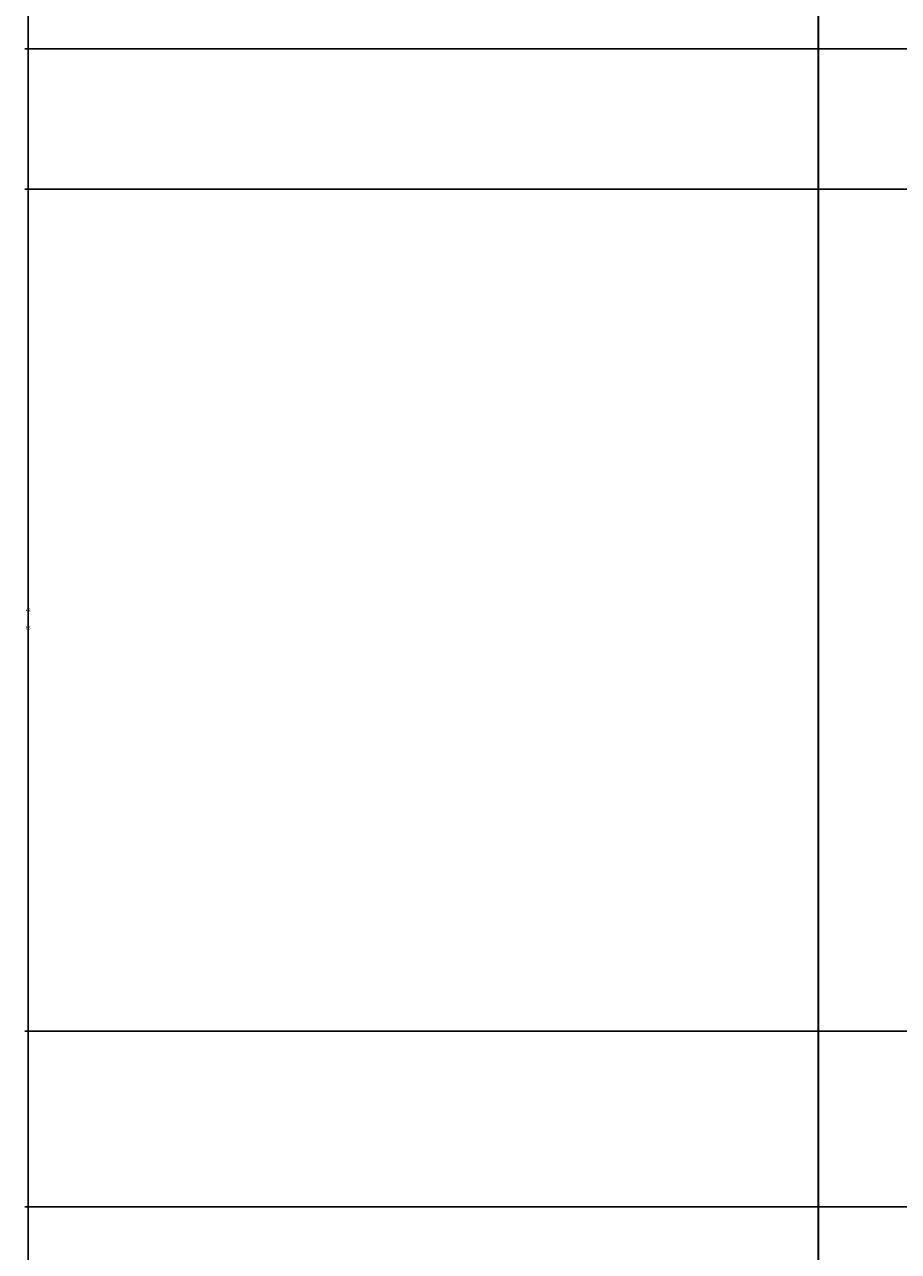
# Model space of a CAD drawing. Units: feet. Extents: x 105 to 1094, y -88 to 588.
# Tile 2 of 59: x 105 to 155, y 138 to 207. Entities that reach past the tile are written whole.
import ezdxf

# ---------------------------------------------------------------- set-up
doc = ezdxf.new("R2010")
doc.units = ezdxf.units.FT
doc.header["$MEASUREMENT"] = 0
doc.layers.add('A-ANNO-DIMS', color=2, linetype='Continuous', lineweight=18)
doc.layers.add('A-WALL', color=7, linetype='Continuous', lineweight=35)
doc.styles.get("Standard").update_dxf_attribs({"font": 'arial.ttf'})
doc.dimstyles.get("Standard").update_dxf_attribs({"dimtxt": 0.18, "dimasz": 0.18, "dimexe": 0.18, "dimexo": 0.0625, "dimgap": 0.09, "dimtad": 0, "dimtih": 1, "dimtoh": 1, "dimdec": 4, "dimzin": 0, "dimdsep": 46, "dimtxsty": 'Standard', "dimcen": 0.09, "dimadec": 0, "dimazin": 0, "dimtfac": 1, "dimtdec": 4, "dimtofl": 0, "dimtmove": 0, "dimatfit": 3, "dimfxl": 1, "dimtolj": 1, "dimtzin": 0, "dimarcsym": 0})

# ---------------------------------------------------------------- blocks, each defined once
blk = doc.blocks.new('*D20')
at = {"layer": 'A-ANNO-DIMS', "color": 0, "lineweight": -2, "transparency": 16777216}
for p, q in [((150.688, 276.019), (150.688, -88.149)), ((1048.688, 276.019), (1048.688, -88.149)), ((150.868, -87.969), (599.399, -87.969)), ((1048.508, -87.969), (599.977, -87.969))]:
    blk.add_line(p, q, dxfattribs=at)
at = {"layer": 'A-ANNO-DIMS', "color": 0, "transparency": 16777216}
for points in [[(150.868, -87.939), (150.868, -87.999), (150.688, -87.969)], [(1048.508, -87.939), (1048.508, -87.999), (1048.688, -87.969)]]:
    blk.add_solid(points, dxfattribs=at)
at = {"layer": 'Defpoints', "color": 0, "transparency": 16777216}
for p in [(150.688, 276.081), (1048.688, 276.081), (1048.688, -87.969)]:
    blk.add_point(p, dxfattribs=at)
at = {"layer": 'A-ANNO-DIMS', "color": 0, "transparency": 16777216, "insert": (599.688, -87.969), "char_height": 0.18, "attachment_point": 5}
blk.add_mtext('\\A1;898', dxfattribs=at)
blk = doc.blocks.new('*D21')
at = {"layer": 'A-ANNO-DIMS', "color": 0, "lineweight": -2, "transparency": 16777216}
for p, q in [((849.626, 543.081), (105.458, 543.081)), ((105.638, 542.901), (105.638, 250.263)), ((105.638, -42.739), (105.638, 249.899)), ((849.626, -42.919), (105.458, -42.919))]:
    blk.add_line(p, q, dxfattribs=at)
at = {"layer": 'A-ANNO-DIMS', "color": 0, "transparency": 16777216}
for points in [[(105.608, 542.901), (105.668, 542.901), (105.638, 543.081)], [(105.608, -42.739), (105.668, -42.739), (105.638, -42.919)]]:
    blk.add_solid(points, dxfattribs=at)
at = {"layer": 'Defpoints', "color": 0, "transparency": 16777216}
for p in [(105.638, 543.081), (849.688, 543.081), (849.688, -42.919)]:
    blk.add_point(p, dxfattribs=at)
at = {"layer": 'A-ANNO-DIMS', "color": 0, "transparency": 16777216, "insert": (105.638, 250.081), "char_height": 0.18, "attachment_point": 5}
blk.add_mtext('\\A1;586', dxfattribs=at)
blk = doc.blocks.new('*D46')
at = {"layer": 'A-ANNO-DIMS', "color": 0, "lineweight": -2, "transparency": 16777216}
for p, q in [((580.626, 206.081), (105.458, 206.081)), ((105.638, 205.901), (105.638, 173.263)), ((105.638, 140.261), (105.638, 172.899)), ((580.626, 140.081), (105.458, 140.081))]:
    blk.add_line(p, q, dxfattribs=at)
at = {"layer": 'A-ANNO-DIMS', "color": 0, "transparency": 16777216}
for points in [[(105.608, 205.901), (105.668, 205.901), (105.638, 206.081)], [(105.608, 140.261), (105.668, 140.261), (105.638, 140.081)]]:
    blk.add_solid(points, dxfattribs=at)
at = {"layer": 'Defpoints', "color": 0, "transparency": 16777216}
for p in [(580.688, 206.081), (105.638, 140.081), (580.688, 140.081)]:
    blk.add_point(p, dxfattribs=at)
at = {"layer": 'A-ANNO-DIMS', "color": 0, "transparency": 16777216, "insert": (105.638, 173.081), "char_height": 0.18, "attachment_point": 5}
blk.add_mtext('\\A1;66', dxfattribs=at)
blk = doc.blocks.new('*D55')
at = {"layer": 'A-ANNO-DIMS', "color": 0, "lineweight": -2, "transparency": 16777216}
for p, q in [((292.626, 198.081), (105.458, 198.081)), ((105.638, 197.901), (105.638, 174.263)), ((105.638, 150.261), (105.638, 173.899)), ((293.134, 150.081), (105.458, 150.081))]:
    blk.add_line(p, q, dxfattribs=at)
at = {"layer": 'A-ANNO-DIMS', "color": 0, "transparency": 16777216}
for points in [[(105.608, 197.901), (105.668, 197.901), (105.638, 198.081)], [(105.608, 150.261), (105.668, 150.261), (105.638, 150.081)]]:
    blk.add_solid(points, dxfattribs=at)
at = {"layer": 'Defpoints', "color": 0, "transparency": 16777216}
for p in [(105.638, 198.081), (292.688, 198.081), (293.197, 150.081)]:
    blk.add_point(p, dxfattribs=at)
at = {"layer": 'A-ANNO-DIMS', "color": 0, "transparency": 16777216, "insert": (105.638, 174.081), "char_height": 0.18, "attachment_point": 5}
blk.add_mtext('\\A1;48', dxfattribs=at)

msp = doc.modelspace()

# ---------------------------------------------------------------- linework, layer by layer
at = {"layer": 'A-WALL'}
msp.add_line((150.6883, 224.0812), (150.6883, 106.0812), dxfattribs=at)

# ---------------------------------------------------------------- dimensions: what is measured, and where the dimension line sits
at = {"layer": 'A-ANNO-DIMS'}
for base, p1, p2, picture, middle in [((105.6383, 543.0812), (849.6883, -42.9188), (849.6883, 543.0812), '*D21', (105.6383, 250.0812)), ((105.6383, 140.0812), (580.6883, 206.0812), (580.6883, 140.0812), '*D46', (105.6383, 173.0812)), ((105.6383, 198.0812), (293.1967, 150.0812), (292.6883, 198.0812), '*D55', (105.6383, 174.0812))]:
    dim = msp.add_linear_dim(base=base, p1=p1, p2=p2, angle=90, dimstyle='Standard', override={"dimdec": 0, "dimlfac": 1, "dimrnd": 0, "dimzin": 0, "dimdsep": 46, "dimlunit": 2}, dxfattribs=at)
    dim.commit()
    dim.dimension.update_dxf_attribs({"geometry": picture, "text_midpoint": middle})
dim = msp.add_linear_dim(base=(1048.6883, -87.9688), p1=(150.6883, 276.0812), p2=(1048.6883, 276.0812), dimstyle='Standard', override={"dimdec": 0, "dimlfac": 1, "dimrnd": 0, "dimzin": 0, "dimdsep": 46, "dimlunit": 2}, dxfattribs=at)
dim.commit()
dim.dimension.update_dxf_attribs({"geometry": '*D20', "text_midpoint": (599.6883, -87.9688)})

doc.saveas('drawing.dxf')
